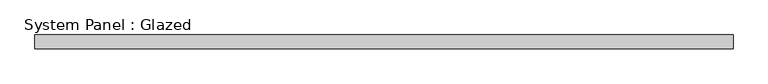
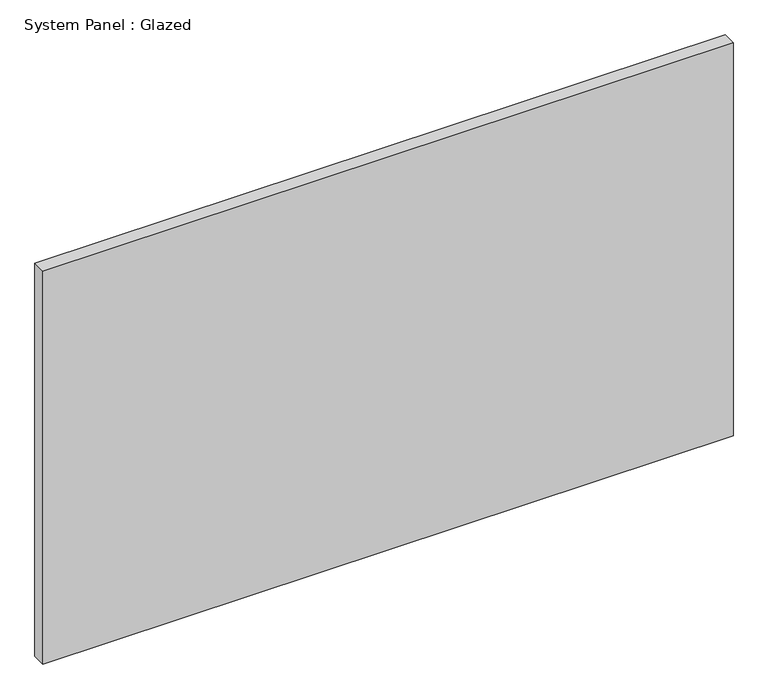
"""IFC4 building model written with IfcOpenShell, lengths in millimetres: plate geometry, System Panel : Glazed."""

from ifc_helpers import new_model, si_unit, origin, origin_with_axes, place, context, project, spatial, polyline, outline, extrude, source, transform, mapped, element, save


def system_panel_glazed_117fd4c3(model_context):
    return source(origin(), model_context, "Body", "SweptSolid", [
        extrude(outline(polyline([(629.7083333, 19.05), (-629.7083333, 19.05), (-629.7083333, 44.45), (629.7083333, 44.45), (629.7083333, 19.05)])), origin_with_axes(), (0.0, 0.0, 1.0), 757.5270145),
    ])


if __name__ == "__main__":
    model = new_model("IFC4")
    model_context = context("Model", 3, world=origin())
    ifc_project = project(units=[si_unit("LENGTHUNIT", "METRE", prefix="MILLI")], contexts=[model_context])
    site = spatial("IfcSite", under=ifc_project)
    building = spatial("IfcBuilding", under=site)
    placement = place(None, origin())
    system_panel_glazed_shape = system_panel_glazed_117fd4c3(model_context)
    element("IfcPlate", 1, ObjectType="System Panel : Glazed", at=placement, inside=building, context=model_context, shape_type="MappedRepresentation", body=[
        mapped(system_panel_glazed_shape, transform((0.0, 0.0, 0.0), x_axis=(1.0, 0.0, 0.0), y_axis=(0.0, 1.0, 0.0), z_axis=(0.0, 0.0, 1.0))),
    ])
    save(model, "model.ifc")

# Revit data of these elements
# Type "System Panel : Glazed"
#   Construction Type Id = "GSP4R"
#   Analytic Construction = "1/8 in Pilkington single glazing"
#   Visual Light Transmittance = 0.9
#   Solar Heat Gain Coefficient = 0.86
#   Heat Transfer Coefficient (U) = 1.18115 BTU/(h·ft²·°F)
#   Define Thermal Properties by = 1
# Element 1 (IfcPlate, "System Panel : Glazed")
#   Materials on its faces: "Glass"
# Materials
#   "Glass": class "Glass", colour RGB 0 128 192, transparency 0.75, Description = "Soda Lime Glass", Cost = 0
